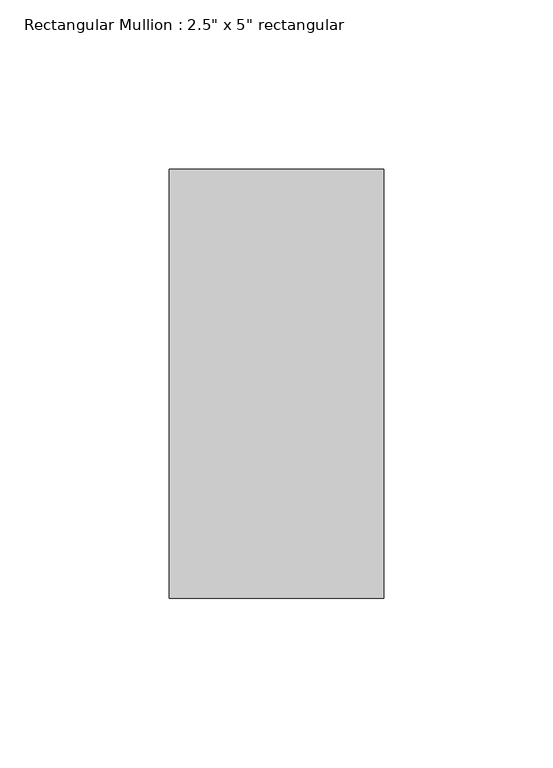
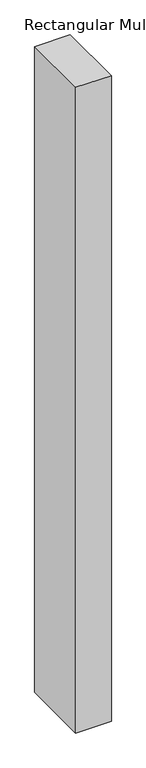
"""IFC4 building model written with IfcOpenShell, lengths in millimetres: member geometry."""

from ifc_helpers import new_model, si_unit, frame, origin, place, context, project, spatial, polyline, outline, extrude, source, transform, mapped, element, save


def member_2b49869a(model_context):
    return source(origin(), model_context, "Body", "SweptSolid", [
        extrude(outline(polyline([(31.75, 63.5), (31.75, -63.5), (-31.75, -63.5), (-31.75, 63.5), (31.75, 63.5)])), frame((0.0, 0.0, -1219.2), z_axis=(0.0, 0.0, 1.0), x_axis=(1.0, 0.0, 0.0)), (0.0, 0.0, 1.0), 1219.2),
    ])


if __name__ == "__main__":
    model = new_model("IFC4")
    model_context = context("Model", 3, world=origin())
    ifc_project = project(units=[si_unit("LENGTHUNIT", "METRE", prefix="MILLI")], contexts=[model_context])
    site = spatial("IfcSite", under=ifc_project)
    building = spatial("IfcBuilding", under=site)
    placement = place(None, origin())
    member_shape = member_2b49869a(model_context)
    element("IfcMember", 1, ObjectType="Rectangular Mullion : 2.5\" x 5\" rectangular", at=placement, inside=building, context=model_context, shape_type="MappedRepresentation", body=[
        mapped(member_shape, transform((0.0, 0.0, 0.0), x_axis=(1.0, 0.0, 0.0), y_axis=(0.0, 1.0, 0.0), z_axis=(0.0, 0.0, 1.0))),
    ])
    save(model, "model.ifc")

# Revit data of these elements
# Type "Rectangular Mullion : 2.5\" x 5\" rectangular"
#   built-in parameter 1007304 = 0.416667 (stored number, unit not read)
#   built-in parameter 1007301 = 0.104167 (stored number, unit not read)
#   built-in parameter 1007300 = 0.104167 (stored number, unit not read)
# Element 1 (IfcMember, "Rectangular Mullion : 2.5\" x 5\" rectangular")
#   Materials on its faces: "Iron, Ductile"
# Materials
#   "Iron, Ductile": class "Metal", colour RGB 0 0 0, transparency 0, Description = "Ductile cast iron", Cost = 0
